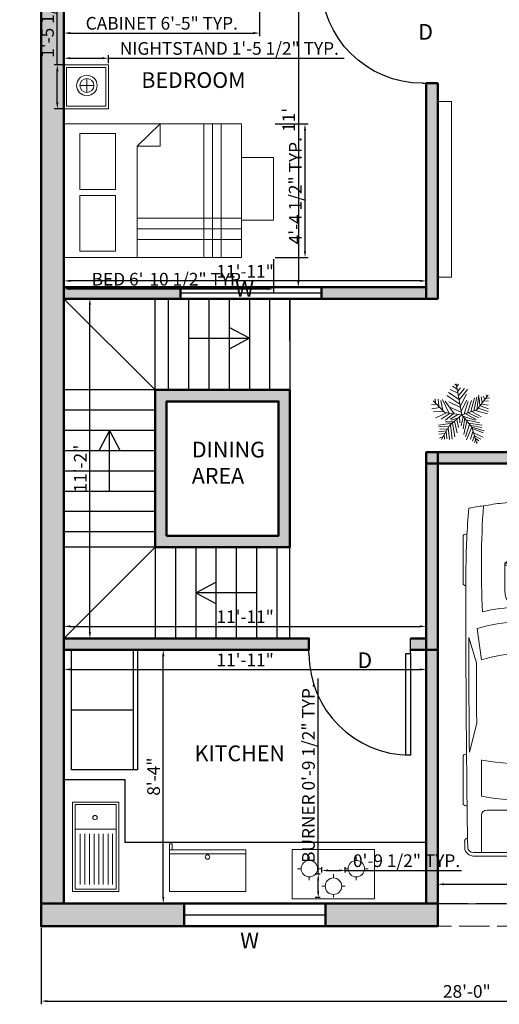
# Model space of a CAD drawing. Units: inches. Extents: x 2227 to 2709, y 1385 to 2029.
# Tile 1 of 4: x 2282 to 2472, y 1385 to 1773. Entities that reach past the tile are written whole.
import ezdxf

# ---------------------------------------------------------------- set-up
doc = ezdxf.new("R2010")
doc.units = ezdxf.units.IN
doc.linetypes.add('ACAD_ISO02W100', pattern=[15, 12, -3])
for name, color, linetype, lineweight in [('A-ANNO-DIMS', 1, 'Continuous', 18), ('A-ANNO-TEXT', 30, 'Continuous', 18), ('A-AREA-IDEN', 30, 'Continuous', 25), ('A-EQPM', 9, 'Continuous', 18), ('A-FLOR-CASE', 50, 'Continuous', 25), ('A-FLOR-FIXT', 9, 'Continuous', 18), ('A-FLOR-STRS', 7, 'Continuous', 25), ('A-FLOR-THRE', 8, 'ACAD_ISO02W100', 18), ('A-FURN', 50, 'Continuous', 18), ('A-SITE-VEHI', 8, 'Continuous', 13), ('A-WALL-PATT', 252, 'Continuous', 13), ('BED', 50, 'Continuous', 18), ('DOOR', 130, 'Continuous', 25), ('TREE', 80, 'Continuous', 13), ('WALL', 160, 'Continuous', 50), ('WIND', 40, 'Continuous', 25)]:
    doc.layers.add(name, color=color, linetype=linetype, lineweight=lineweight)
doc.styles.get("Standard").update_dxf_attribs({"font": 'arial.ttf'})
doc.dimstyles.new('ISO-25', dxfattribs={"dimtxt": 5, "dimasz": 2.5, "dimexe": 1.25, "dimexo": 0.625, "dimtad": 1, "dimdec": 0, "dimlunit": 4, "dimtxsty": 'Standard', "dimcen": 2.5, "dimadec": 0, "dimazin": 0, "dimtfac": 1, "dimtdec": 0, "dimtmove": 0, "dimatfit": 3, "dimfxl": 1, "dimarcsym": 0})

# ---------------------------------------------------------------- blocks, each defined once
blk = doc.blocks.new('*U8')
for p, q in [((21.1, 37.41), (21.1, 36.83)), ((46.55, 38.89), (22.35, 38.89)), ((47.8, 37.39), (47.8, 37.41)), ((87.99, 31.87), (74.76, 35.92)), ((135.45, 37.07), (135.45, 37.41)), ((136.7, 38.89), (160.9, 38.89)), ((162.15, 37.41), (162.15, 36.77)), ((70.03, 31.54), (86.41, 29.35)), ((134.31, 35.6), (119.29, 31.78)), ((186.47, -33.5), (186.47, 33.5)), ((188.4, -32.76), (188.4, 32.76)), ((138.42, 29.35), (157.25, 29.35)), ((164.52, 26.39), (164.52, -26.39)), ((186.47, 29.35), (167.01, 29.35)), ((32.27, 11.63), (36.13, 17.17)), ((36.13, 17.17), (50.94, 17.17)), ((32.12, 9.51), (32.12, 11.15)), ((58.92, -10.77), (58.92, 10.77)), ((66.55, -10.53), (66.55, 10.53)), ((186.47, -10.53), (186.47, 10.53)), ((3.27, 6.13), (0.1, 0.41)), ((29.77, 9.51), (51.68, 9.51)), ((82.74, 8.5), (82.74, -8.5)), ((0, 0), (51.68, 0)), ((0.1, -0.41), (3.27, -6.13)), ((29.77, -9.51), (51.68, -9.51)), ((32.12, -9.51), (32.12, -11.15)), ((32.27, -11.63), (36.13, -17.17)), ((36.13, -17.17), (50.94, -17.17)), ((86.41, -29.35), (70.03, -31.54)), ((157.25, -29.35), (138.42, -29.35)), ((167.01, -29.35), (186.47, -29.35)), ((87.99, -31.87), (74.76, -35.92)), ((134.31, -35.6), (119.29, -31.78)), ((21.1, -37.41), (21.1, -36.83)), ((46.55, -38.89), (22.35, -38.89)), ((47.8, -37.39), (47.8, -37.41)), ((135.45, -37.07), (135.45, -37.41)), ((136.7, -38.89), (160.9, -38.89)), ((162.15, -37.41), (162.15, -36.77))]:
    blk.add_line(p, q)
for centre, major_axis, ratio, start_param, end_param in [((266.03, -27.52), (0, 313.31), 0.842304, 1.367076, 1.39176), ((41.19, -490.86), (0, 528.23), 0.842304, 0.00281, 0.075598), ((22.35, 37.41), (0, -1.48), 0.842304, 3.141593, 4.712389), ((64.48, -10555.62), (0, 10593.03), 0.842304, -0.013397, 0.002797), ((46.55, 37.41), (0, 1.48), 0.842304, -1.570796, 0), ((64.48, -10555.62), (0, -10591.55), 0.842304, 3.133765, 3.140441), ((136.7, 37.41), (0, -1.48), 0.842304, 3.141593, 4.712389), ((160.9, 37.41), (0, 1.48), 0.842304, -1.570796, 0), ((180.63, 35.84), (0, 2.22), 0.842304, -0.013017, 1.249894), ((64.48, -10556.36), (0, 10595.31), 0.842304, -0.013397, -0.013017), ((183.98, 33.5), (0, -2.96), 0.842304, 1.570796, 3.128196), ((183.98, 32.76), (0, -5.25), 0.842304, 1.570796, 3.128196), ((135.29, 5.39), (0, 81.77), 0.842304, 1.245306, 1.50788), ((95.79, -3666.35), (0, -3698.24), 0.842304, 3.134049, 3.144098), ((259.18, -27.52), (0, -305.3), 0.842304, 4.528606, 4.561838), ((37.47, -593.96), (0, -623.33), 0.842304, 3.096046, 3.200911), ((134.4, 5.39), (0, -89.78), 0.842304, 4.449482, 4.652344), ((149.6, 2.8), (0, -79.58), 0.842304, 4.372215, 4.640744), ((17.08, 0), (0, 147.02), 0.842304, 4.511394, 4.913384), ((35.91, 0), (0, 147.02), 0.842304, 4.511394, 4.913384), ((167.01, 26.39), (0, 2.96), 0.842304, 0, 1.570796), ((-204.49, 52.4), (0, -250.96), 0.842304, 1.385369, 1.434372), ((13.04, 17.01), (0, 27.42), 0.842304, 4.435146, 4.718221), ((14.2, 17.01), (0, 27.42), 0.842304, 4.435146, 4.718221), ((50.79, 13.34), (6.34, -0.36), 0.603834, -1.395552, 1.581315), ((32.75, 11.15), (0, 0.74), 0.842304, 0.879714, 1.570796), ((29.77, -46.66), (0, 56.17), 0.842304, 0, 0.590319), ((0.62, 0), (0, -0.74), 0.842304, 4.131459, 5.293319), ((29.77, 46.66), (0, 56.17), 0.842304, 2.551274, 3.141593), ((-204.49, -52.4), (0, 250.96), 0.842304, -1.434372, -1.385369), ((13.04, -17.01), (0, -27.42), 0.842304, 1.564964, 1.848039), ((14.2, -17.01), (0, -27.42), 0.842304, 1.564964, 1.848039), ((149.6, -2.8), (0, -79.58), 0.842304, -1.499151, -1.230623), ((32.75, -11.15), (0, -0.74), 0.842304, 4.712389, 5.403472), ((134.4, -5.39), (0, -89.78), 0.842304, -1.510751, -1.307889), ((135.29, -5.39), (0, -81.77), 0.842304, -1.50788, -1.245306), ((259.18, 27.52), (0, 305.3), 0.842304, 1.721348, 1.754579), ((266.03, 27.52), (0, 313.31), 0.842304, 1.749832, 1.774517), ((37.47, 593.96), (0, -623.33), 0.842304, -0.059319, 0.045547), ((167.01, -26.39), (0, -2.96), 0.842304, 4.712389, 6.283185), ((64.48, 10555.62), (0, -10591.55), 0.842304, 0.001152, 0.007828), ((95.79, 3666.35), (0, -3698.24), 0.842304, -0.002505, 0.007544), ((183.98, -33.5), (0, 2.96), 0.842304, 3.15499, 4.712389), ((183.98, -32.76), (0, -5.25), 0.842304, 0.013397, 1.570796), ((41.19, 490.86), (0, -528.23), 0.842304, -0.075598, -0.00281), ((22.35, -37.41), (0, 1.48), 0.842304, 1.570796, 3.141593), ((64.48, 10555.62), (0, 10593.03), 0.842304, 3.138796, 3.15499), ((46.55, -37.41), (0, -1.48), 0.842304, 0, 1.570796), ((136.7, -37.41), (0, -1.48), 0.842304, -1.570796, 0), ((160.9, -37.41), (0, 1.48), 0.842304, 3.141593, 4.712389), ((180.63, -35.84), (0, -2.22), 0.842304, -1.249894, 0.013017), ((64.48, 10556.36), (0, 10595.31), 0.842304, 3.15461, 3.15499)]:
    blk.add_ellipse(centre, major_axis=major_axis, ratio=ratio, start_param=start_param, end_param=end_param)
at = {"extrusion": (0, 0, -1)}
blk.add_ellipse((50.79, -13.34), major_axis=(6.34, 0.36), ratio=0.603834, start_param=-1.395552, end_param=1.581315, dxfattribs=at)
blk = doc.blocks.new('*U2')
for p, q in [((0, 0), (0, -6)), ((40, 0), (40, -6))]:
    blk.add_line(p, q)
blk.add_lwpolyline([(0, 0), (0, 40), (1.75, 40), (1.75, 0)], close=True)
blk.add_arc((0, 0), 40, 0, 90)
blk = doc.blocks.new('*U6')
for p, q in [((-10.186, 53.64), (-13.084, 55.962)), ((0, 0), (-10.5, 57)), ((-9.099, 51.782), (-6.563, 55.962)), ((-5.114, 28.097), (-24.676, 40.636)), ((-7.288, 39.707), (-21.778, 46.673)), ((-8.737, 47.138), (-17.069, 52.711)), ((-7.65, 43.423), (-2.578, 49.46)), ((-5.839, 35.992), (4.667, 48.067)), ((-5.114, 27.632), (10.463, 46.673)), ((-2.941, 16.486), (8.652, 37.85)), ((44.153, 36.456), (45.239, 32.741)), ((-47.498, 19.737), (-55.83, 18.344)), ((-31.5, 4.5), (-52.5, 25.5)), ((-48.585, 21.131), (-49.309, 29.026)), ((-43.513, 28.561), (-42.427, 15.558)), ((-38.442, 26.239), (-34.819, 7.663)), ((-35.544, 28.097), (-24.314, 3.947)), ((-14.533, 2.09), (-30.834, 25.31)), ((-3.665, 19.273), (-27.574, 35.527)), ((-24.314, 23.917), (-2.941, 13.7)), ((-1.129, 6.734), (9.014, 26.704)), ((3.942, 1.625), (11.187, 24.381)), ((10.101, 3.483), (17.708, 26.239)), ((16.259, 5.805), (23.142, 31.348)), ((22.055, 7.198), (27.489, 32.277)), ((27, 9), (48, 36)), ((27.127, 9.056), (31.112, 35.992)), ((31.836, 30.883), (32.561, 16.486)), ((35.096, 32.741), (37.27, 22.524)), ((36.183, 19.737), (48.137, 17.88)), ((38.719, 34.134), (41.979, 28.561)), ((40.53, 25.775), (48.862, 24.846)), ((43.791, 29.954), (51.036, 30.883)), ((-40.615, 13.7), (-55.105, 10.913)), ((-33.37, 6.269), (-52.207, 5.34)), ((-28.299, 3.483), (-47.86, -5.805)), ((-21.416, 3.018), (-38.079, -8.128)), ((0, 0), (-31.5, 4.5)), ((-15.982, 2.09), (-30.11, -9.521)), ((0, 0), (-22.5, -19.5)), ((-6.563, 1.161), (-21.416, -8.128)), ((-20.691, 13.7), (-1.129, 4.876)), ((0, 0), (27, 9)), ((0, 0), (18, -22.5)), ((6.478, 1.625), (26.04, -8.592)), ((11.187, 3.483), (30.749, -5.805)), ((18.07, 5.805), (35.096, -3.483)), ((24.229, 7.663), (46.688, 1.625)), ((29.662, 12.307), (48.137, 6.269)), ((33.285, 16.486), (48.862, 10.913)), ((-17.431, -15.094), (-42.789, -18.809)), ((-15.257, -12.772), (-30.11, -12.772)), ((-6.563, -5.805), (-19.967, -9.985)), ((-17.069, -15.094), (-12.721, -40.172)), ((-13.446, -11.378), (-8.737, -32.741)), ((-9.461, -8.592), (-6.201, -23.453)), ((-4.752, -3.483), (-3.665, -14.629)), ((2.493, -3.019), (-1.491, -20.202)), ((1.769, -2.555), (24.229, -9.521)), ((5.029, -6.27), (2.131, -25.775)), ((9.014, -11.378), (3.58, -35.992)), ((14.085, -16.951), (6.478, -40.172)), ((7.565, -9.056), (32.198, -14.629)), ((12.274, -15.094), (36.907, -18.809)), ((-28.299, -29.026), (-42.789, -31.348)), ((-24.314, -21.596), (-42.427, -22.06)), ((-30.834, -34.135), (-42.427, -35.528)), ((-26.849, -26.24), (-40.253, -25.775)), ((-22.5, -19.5), (-37.5, -45)), ((-29.023, -30.884), (-27.936, -43.887)), ((-25.038, -23.918), (-22.865, -45.281)), ((-20.691, -18.345), (-17.793, -44.352)), ((18.07, -22.524), (8.289, -45.745)), ((20.244, -30.419), (15.897, -44.816)), ((16.259, -19.738), (36.183, -22.989)), ((18, -22.5), (27, -52.5)), ((18.433, -22.524), (40.53, -29.026)), ((19.157, -25.311), (38.719, -33.206)), ((21.331, -32.741), (39.081, -40.636)), ((-34.457, -39.708), (-40.978, -42.494)), ((-32.646, -36.921), (-31.921, -44.352)), ((22.78, -37.85), (19.519, -48.532)), ((22.78, -38.314), (34.372, -44.816)), ((24.591, -45.745), (23.142, -50.854)), ((24.591, -43.423), (30.749, -47.603)), ((26.764, -49.925), (28.213, -50.854))]:
    blk.add_line(p, q)
blk = doc.blocks.new('*D21')
at = {"layer": 'A-ANNO-DIMS', "color": 0, "lineweight": -2, "transparency": 16777216}
for p, q in [((2300.34, 1799.33), (2393.46, 1799.33)), ((2392.21, 1796.83), (2392.21, 1669.83)), ((2300.34, 1667.33), (2393.46, 1667.33))]:
    blk.add_line(p, q, dxfattribs=at)
at = {"layer": 'A-ANNO-DIMS', "color": 0, "lineweight": 100, "transparency": 16777216}
for points in [[(2391.79, 1796.83), (2392.62, 1796.83), (2392.21, 1799.33)], [(2391.79, 1669.83), (2392.62, 1669.83), (2392.21, 1667.33)]]:
    blk.add_solid(points, dxfattribs=at)
at = {"layer": 'Defpoints', "color": 0, "lineweight": 100, "transparency": 16777216}
for p in [(2299.71, 1799.33), (2299.71, 1667.33), (2392.21, 1667.33)]:
    blk.add_point(p, dxfattribs=at)
at = {"layer": 'A-ANNO-DIMS', "color": 0, "transparency": 16777216, "insert": (2389.07, 1733.33), "char_height": 5, "attachment_point": 5, "rotation": 90}
blk.add_mtext("11'", dxfattribs=at)
blk = doc.blocks.new('*D22')
at = {"layer": 'A-ANNO-DIMS', "color": 0, "lineweight": -2, "transparency": 16777216}
for p, q in [((2299.71, 1667.96), (2299.71, 1671.09)), ((2440.21, 1669.84), (2302.21, 1669.84)), ((2442.71, 1667.96), (2442.71, 1671.09))]:
    blk.add_line(p, q, dxfattribs=at)
at = {"layer": 'A-ANNO-DIMS', "color": 0, "lineweight": 100, "transparency": 16777216}
for points in [[(2302.21, 1670.26), (2302.21, 1669.42), (2299.71, 1669.84)], [(2440.21, 1670.26), (2440.21, 1669.42), (2442.71, 1669.84)]]:
    blk.add_solid(points, dxfattribs=at)
at = {"layer": 'Defpoints', "color": 0, "lineweight": 100, "transparency": 16777216}
for p in [(2299.71, 1669.84), (2299.71, 1667.33), (2442.71, 1667.33)]:
    blk.add_point(p, dxfattribs=at)
at = {"layer": 'A-ANNO-DIMS', "color": 0, "transparency": 16777216, "insert": (2371.21, 1672.98), "char_height": 5, "attachment_point": 5}
blk.add_mtext('11\'-11"', dxfattribs=at)
blk = doc.blocks.new('*D23')
at = {"layer": 'A-ANNO-DIMS', "color": 0, "lineweight": -2, "transparency": 16777216}
for p, q in [((2300.34, 1662.83), (2311.19, 1662.83)), ((2309.94, 1531.33), (2309.94, 1660.33)), ((2300.34, 1528.83), (2311.19, 1528.83))]:
    blk.add_line(p, q, dxfattribs=at)
at = {"layer": 'A-ANNO-DIMS', "color": 0, "lineweight": 100, "transparency": 16777216}
for points in [[(2309.52, 1660.33), (2310.35, 1660.33), (2309.94, 1662.83)], [(2309.52, 1531.33), (2310.35, 1531.33), (2309.94, 1528.83)]]:
    blk.add_solid(points, dxfattribs=at)
at = {"layer": 'Defpoints', "color": 0, "lineweight": 100, "transparency": 16777216}
for p in [(2299.71, 1662.83), (2309.94, 1662.83), (2299.71, 1528.83)]:
    blk.add_point(p, dxfattribs=at)
at = {"layer": 'A-ANNO-DIMS', "color": 0, "transparency": 16777216, "insert": (2306.8, 1595.83), "char_height": 5, "attachment_point": 5, "rotation": 90}
blk.add_mtext('11\'-2"', dxfattribs=at)
blk = doc.blocks.new('*D24')
at = {"layer": 'A-ANNO-DIMS', "color": 0, "lineweight": -2, "transparency": 16777216}
for p, q in [((2299.71, 1529.46), (2299.71, 1534.84)), ((2442.71, 1529.46), (2442.71, 1534.84)), ((2302.21, 1533.59), (2440.21, 1533.59))]:
    blk.add_line(p, q, dxfattribs=at)
at = {"layer": 'A-ANNO-DIMS', "color": 0, "lineweight": 100, "transparency": 16777216}
for points in [[(2302.21, 1534.01), (2302.21, 1533.18), (2299.71, 1533.59)], [(2440.21, 1534.01), (2440.21, 1533.18), (2442.71, 1533.59)]]:
    blk.add_solid(points, dxfattribs=at)
at = {"layer": 'Defpoints', "color": 0, "lineweight": 100, "transparency": 16777216}
for p in [(2442.71, 1533.59), (2299.71, 1528.83), (2442.71, 1528.83)]:
    blk.add_point(p, dxfattribs=at)
at = {"layer": 'A-ANNO-DIMS', "color": 0, "transparency": 16777216, "insert": (2371.21, 1536.73), "char_height": 5, "attachment_point": 5}
blk.add_mtext('11\'-11"', dxfattribs=at)
blk = doc.blocks.new('*D25')
at = {"layer": 'A-ANNO-DIMS', "color": 0, "lineweight": -2, "transparency": 16777216}
for p, q in [((2299.71, 1523.71), (2299.71, 1515.35)), ((2442.71, 1523.71), (2442.71, 1515.35)), ((2302.21, 1516.6), (2440.21, 1516.6))]:
    blk.add_line(p, q, dxfattribs=at)
at = {"layer": 'A-ANNO-DIMS', "color": 0, "lineweight": 100, "transparency": 16777216}
for points in [[(2302.21, 1517.02), (2302.21, 1516.18), (2299.71, 1516.6)], [(2440.21, 1517.02), (2440.21, 1516.18), (2442.71, 1516.6)]]:
    blk.add_solid(points, dxfattribs=at)
at = {"layer": 'Defpoints', "color": 0, "lineweight": 100, "transparency": 16777216}
for p in [(2299.71, 1524.33), (2442.71, 1524.33), (2442.71, 1516.6)]:
    blk.add_point(p, dxfattribs=at)
at = {"layer": 'A-ANNO-DIMS', "color": 0, "transparency": 16777216, "insert": (2371.21, 1519.74), "char_height": 5, "attachment_point": 5}
blk.add_mtext('11\'-11"', dxfattribs=at)
blk = doc.blocks.new('*D26')
at = {"layer": 'A-ANNO-DIMS', "color": 0, "lineweight": -2, "transparency": 16777216}
for p, q in [((2300.34, 1524.33), (2340.16, 1524.33)), ((2338.91, 1426.83), (2338.91, 1521.83)), ((2300.34, 1424.33), (2340.16, 1424.33))]:
    blk.add_line(p, q, dxfattribs=at)
at = {"layer": 'A-ANNO-DIMS', "color": 0, "lineweight": 100, "transparency": 16777216}
for points in [[(2338.49, 1521.83), (2339.33, 1521.83), (2338.91, 1524.33)], [(2338.49, 1426.83), (2339.33, 1426.83), (2338.91, 1424.33)]]:
    blk.add_solid(points, dxfattribs=at)
at = {"layer": 'Defpoints', "color": 0, "lineweight": 100, "transparency": 16777216}
for p in [(2299.71, 1524.33), (2338.91, 1524.33), (2299.71, 1424.33)]:
    blk.add_point(p, dxfattribs=at)
at = {"layer": 'A-ANNO-DIMS', "color": 0, "transparency": 16777216, "insert": (2335.73, 1474.33), "char_height": 5, "attachment_point": 5, "rotation": 90}
blk.add_mtext('8\'-4"', dxfattribs=at)
blk = doc.blocks.new('*D27')
at = {"layer": 'A-ANNO-DIMS', "color": 0, "lineweight": -2, "transparency": 16777216}
for p, q in [((2447.21, 1424.96), (2447.21, 1433.13)), ((2617.71, 1424.96), (2617.71, 1433.13)), ((2449.71, 1431.88), (2615.21, 1431.88))]:
    blk.add_line(p, q, dxfattribs=at)
at = {"layer": 'A-ANNO-DIMS', "color": 0, "lineweight": 100, "transparency": 16777216}
for points in [[(2449.71, 1432.3), (2449.71, 1431.46), (2447.21, 1431.88)], [(2615.21, 1432.3), (2615.21, 1431.46), (2617.71, 1431.88)]]:
    blk.add_solid(points, dxfattribs=at)
at = {"layer": 'Defpoints', "color": 0, "lineweight": 100, "transparency": 16777216}
for p in [(2617.71, 1431.88), (2447.21, 1424.33), (2617.71, 1424.33)]:
    blk.add_point(p, dxfattribs=at)
at = {"layer": 'A-ANNO-DIMS', "color": 0, "transparency": 16777216, "insert": (2532.46, 1435.06), "char_height": 5, "attachment_point": 5}
blk.add_mtext('14\'-3"', dxfattribs=at)
blk = doc.blocks.new('*D28')
at = {"layer": 'A-ANNO-DIMS', "color": 0, "lineweight": -2, "transparency": 16777216}
for p, q in [((2448.57, 1597.83), (2527.6, 1597.5)), ((2525.63, 1426.5), (2526.34, 1595)), ((2447.84, 1424.33), (2526.87, 1424))]:
    blk.add_line(p, q, dxfattribs=at)
at = {"layer": 'A-ANNO-DIMS', "color": 0, "lineweight": 100, "transparency": 16777216}
for points in [[(2525.92, 1595), (2526.75, 1595), (2526.35, 1597.5)], [(2525.21, 1426.5), (2526.04, 1426.5), (2525.62, 1424)]]:
    blk.add_solid(points, dxfattribs=at)
at = {"layer": 'Defpoints', "color": 0, "lineweight": 100, "transparency": 16777216}
for p in [(2447.95, 1597.83), (2526.35, 1597.5), (2447.21, 1424.33)]:
    blk.add_point(p, dxfattribs=at)
at = {"layer": 'A-ANNO-DIMS', "color": 0, "transparency": 16777216, "insert": (2522.8, 1510.77), "char_height": 5, "attachment_point": 5, "rotation": 89.7584}
blk.add_mtext('14\'-6"', dxfattribs=at)
blk = doc.blocks.new('BED-DOUBLE')
for p, q in [((37.96, 0), (28.86, -8.71)), ((37.96, -8.71), (37.96, 0)), ((55.17, -52.67), (55.17, 0)), ((58.68, -52.67), (58.68, 0)), ((62.04, -52.67), (62.04, 0)), ((28.86, -52.67), (28.86, -8.71)), ((28.86, -8.71), (37.96, -8.71)), ((28.86, -37.1), (70.02, -37.1)), ((28.86, -41.31), (70.02, -41.31)), ((28.86, -45.51), (70.02, -45.51))]:
    blk.add_line(p, q)
for points in [[(0, 0), (70.02, 0), (70.02, -52.67), (0, -52.67)], [(6.26, -25.79), (20.3, -25.79), (20.3, -3.78), (6.26, -3.78)], [(70.02, -38), (82.72, -38), (82.72, -13.23), (70.02, -13.23)], [(6.26, -50.18), (20.3, -50.18), (20.3, -28.17), (6.26, -28.17)]]:
    blk.add_lwpolyline(points, close=True)
blk = doc.blocks.new('NIGHTSTAND')
for p, q in [((9.06, 6.42), (9.06, 11.97)), ((6.28, 9.2), (11.83, 9.2))]:
    blk.add_line(p, q)
for points in [[(0, 0), (17.54, 0), (17.54, 17.32), (0, 17.32)], [(1, 1), (16.54, 1), (16.54, 16.32), (1, 16.32)]]:
    blk.add_lwpolyline(points, close=True)
for radius in [4.05, 2.77]:
    blk.add_circle((9.06, 9.2), radius)
blk = doc.blocks.new('STAIR-DIRECTION')
for p, q in [((0, 0), (8, 4.23)), ((24, 0), (0, 0)), ((0, 0), (8, -4.23))]:
    blk.add_line(p, q)
blk = doc.blocks.new('COOKTOP-BURNER')
for p, q in [((0, 3.25), (0, 4.8)), ((-3.25, 0), (-4.62, 0)), ((0, -3.25), (0, -4.52)), ((3.25, 0), (4.66, 0))]:
    blk.add_line(p, q)
blk.add_circle((0, 0), 3.25)
blk = doc.blocks.new('*D37')
at = {"layer": 'A-ANNO-DIMS', "color": 0, "lineweight": -2, "transparency": 16777216}
for p, q in [((2299.71, 1678.44), (2299.71, 1665.41)), ((2382.43, 1678.44), (2382.43, 1665.41)), ((2302.21, 1666.66), (2379.93, 1666.66))]:
    blk.add_line(p, q, dxfattribs=at)
at = {"layer": 'A-ANNO-DIMS', "color": 0, "lineweight": 100, "transparency": 16777216}
for points in [[(2302.21, 1667.07), (2302.21, 1666.24), (2299.71, 1666.66)], [(2379.93, 1667.07), (2379.93, 1666.24), (2382.43, 1666.66)]]:
    blk.add_solid(points, dxfattribs=at)
at = {"layer": 'Defpoints', "color": 0, "lineweight": 100, "transparency": 16777216}
for p in [(2299.71, 1679.06), (2382.43, 1679.06), (2382.43, 1666.66)]:
    blk.add_point(p, dxfattribs=at)
at = {"layer": 'A-ANNO-DIMS', "color": 0, "transparency": 16777216, "insert": (2341.07, 1669.87), "char_height": 5, "attachment_point": 5}
blk.add_mtext('BED 6\'-10 1/2" TYP.', dxfattribs=at)
blk = doc.blocks.new('*D38')
at = {"layer": 'A-ANNO-DIMS', "color": 0, "lineweight": -2, "transparency": 16777216}
for p, q in [((2383.06, 1731.73), (2396.09, 1731.73)), ((2394.84, 1681.56), (2394.84, 1729.23)), ((2383.06, 1679.06), (2396.09, 1679.06))]:
    blk.add_line(p, q, dxfattribs=at)
at = {"layer": 'A-ANNO-DIMS', "color": 0, "lineweight": 100, "transparency": 16777216}
for points in [[(2394.42, 1729.23), (2395.25, 1729.23), (2394.84, 1731.73)], [(2394.42, 1681.56), (2395.25, 1681.56), (2394.84, 1679.06)]]:
    blk.add_solid(points, dxfattribs=at)
at = {"layer": 'Defpoints', "color": 0, "lineweight": 100, "transparency": 16777216}
for p in [(2382.43, 1731.73), (2394.84, 1731.73), (2382.43, 1679.06)]:
    blk.add_point(p, dxfattribs=at)
at = {"layer": 'A-ANNO-DIMS', "color": 0, "transparency": 16777216, "insert": (2391.63, 1705.4), "char_height": 5, "attachment_point": 5, "rotation": 90}
blk.add_mtext('4\'-4 1/2" TYP.', dxfattribs=at)
blk = doc.blocks.new('*D39')
at = {"layer": 'A-ANNO-DIMS', "color": 0, "lineweight": -2, "transparency": 16777216}
for p, q in [((2299.71, 1778.54), (2299.71, 1766.33)), ((2376.93, 1778.54), (2376.93, 1766.33)), ((2302.21, 1767.58), (2374.43, 1767.58))]:
    blk.add_line(p, q, dxfattribs=at)
at = {"layer": 'A-ANNO-DIMS', "color": 0, "lineweight": 100, "transparency": 16777216}
for points in [[(2302.21, 1768), (2302.21, 1767.16), (2299.71, 1767.58)], [(2374.43, 1768), (2374.43, 1767.16), (2376.93, 1767.58)]]:
    blk.add_solid(points, dxfattribs=at)
at = {"layer": 'Defpoints', "color": 0, "lineweight": 100, "transparency": 16777216}
for p in [(2299.71, 1779.16), (2376.93, 1779.16), (2376.93, 1767.58)]:
    blk.add_point(p, dxfattribs=at)
at = {"layer": 'A-ANNO-DIMS', "color": 0, "transparency": 16777216, "insert": (2338.32, 1770.79), "char_height": 5, "attachment_point": 5}
blk.add_mtext('CABINET 6\'-5" TYP.', dxfattribs=at)
blk = doc.blocks.new('*D41')
at = {"layer": 'A-ANNO-DIMS', "color": 0, "lineweight": -2, "transparency": 16777216}
for p, q in [((2299.71, 1755.65), (2299.71, 1758.91)), ((2302.21, 1757.66), (2314.75, 1757.66)), ((2317.25, 1755.65), (2317.25, 1758.91)), ((2317.25, 1757.66), (2410.23, 1757.66))]:
    blk.add_line(p, q, dxfattribs=at)
at = {"layer": 'A-ANNO-DIMS', "color": 0, "lineweight": 100, "transparency": 16777216}
for points in [[(2302.21, 1758.07), (2302.21, 1757.24), (2299.71, 1757.66)], [(2314.75, 1758.07), (2314.75, 1757.24), (2317.25, 1757.66)]]:
    blk.add_solid(points, dxfattribs=at)
at = {"layer": 'Defpoints', "color": 0, "lineweight": 100, "transparency": 16777216}
for p in [(2317.25, 1757.66), (2299.71, 1755.03), (2317.25, 1755.03)]:
    blk.add_point(p, dxfattribs=at)
at = {"layer": 'A-ANNO-DIMS', "color": 0, "transparency": 16777216, "insert": (2364.99, 1760.87), "char_height": 5, "attachment_point": 5}
blk.add_mtext('NIGHTSTAND 1\'-5 1/2" TYP.', dxfattribs=at)
blk = doc.blocks.new('*D42')
at = {"layer": 'A-ANNO-DIMS', "color": 0, "lineweight": -2, "transparency": 16777216}
for p, q in [((2297.08, 1755.03), (2297.08, 1800.43)), ((2299.09, 1755.03), (2295.83, 1755.03)), ((2297.08, 1740.21), (2297.08, 1752.53)), ((2299.09, 1737.71), (2295.83, 1737.71))]:
    blk.add_line(p, q, dxfattribs=at)
at = {"layer": 'A-ANNO-DIMS', "color": 0, "lineweight": 100, "transparency": 16777216}
for points in [[(2296.67, 1752.53), (2297.5, 1752.53), (2297.08, 1755.03)], [(2296.67, 1740.21), (2297.5, 1740.21), (2297.08, 1737.71)]]:
    blk.add_solid(points, dxfattribs=at)
at = {"layer": 'Defpoints', "color": 0, "lineweight": 100, "transparency": 16777216}
for p in [(2297.08, 1755.03), (2299.71, 1755.03), (2299.71, 1737.71)]:
    blk.add_point(p, dxfattribs=at)
at = {"layer": 'A-ANNO-DIMS', "color": 0, "transparency": 16777216, "insert": (2293.87, 1778.98), "char_height": 5, "attachment_point": 5, "rotation": 90}
blk.add_mtext('1\'-5 1/2" TYP.', dxfattribs=at)
blk = doc.blocks.new('*D45')
at = {"layer": 'A-ANNO-DIMS', "color": 0, "lineweight": -2, "transparency": 16777216}
for p, q in [((2400.05, 1435.92), (2400.05, 1513.02)), ((2400.82, 1435.92), (2398.8, 1435.92)), ((2400.05, 1429.1), (2400.05, 1433.42)), ((2400.82, 1426.6), (2398.8, 1426.6))]:
    blk.add_line(p, q, dxfattribs=at)
at = {"layer": 'A-ANNO-DIMS', "color": 0, "lineweight": 100, "transparency": 16777216}
for points in [[(2399.63, 1433.42), (2400.46, 1433.42), (2400.05, 1435.92)], [(2399.63, 1429.1), (2400.46, 1429.1), (2400.05, 1426.6)]]:
    blk.add_solid(points, dxfattribs=at)
at = {"layer": 'Defpoints', "color": 0, "lineweight": 100, "transparency": 16777216}
for p in [(2400.05, 1435.92), (2401.45, 1435.92), (2401.45, 1426.6)]:
    blk.add_point(p, dxfattribs=at)
at = {"layer": 'A-ANNO-DIMS', "color": 0, "transparency": 16777216, "insert": (2396.84, 1475.72), "char_height": 5, "attachment_point": 5, "rotation": 90}
blk.add_mtext('BURNER 0\'-9 1/2" TYP.', dxfattribs=at)
blk = doc.blocks.new('*D46')
at = {"layer": 'A-ANNO-DIMS', "color": 0, "lineweight": -2, "transparency": 16777216}
for p, q in [((2401.45, 1436.55), (2401.45, 1438.57)), ((2403.95, 1437.32), (2408.23, 1437.32)), ((2410.73, 1436.55), (2410.73, 1438.57)), ((2410.73, 1437.32), (2456.61, 1437.32))]:
    blk.add_line(p, q, dxfattribs=at)
at = {"layer": 'A-ANNO-DIMS', "color": 0, "lineweight": 100, "transparency": 16777216}
for points in [[(2403.95, 1437.74), (2403.95, 1436.91), (2401.45, 1437.32)], [(2408.23, 1437.74), (2408.23, 1436.91), (2410.73, 1437.32)]]:
    blk.add_solid(points, dxfattribs=at)
at = {"layer": 'Defpoints', "color": 0, "lineweight": 100, "transparency": 16777216}
for p in [(2410.73, 1437.32), (2401.45, 1435.92), (2410.73, 1435.92)]:
    blk.add_point(p, dxfattribs=at)
at = {"layer": 'A-ANNO-DIMS', "color": 0, "transparency": 16777216, "insert": (2434.92, 1440.53), "char_height": 5, "attachment_point": 5}
blk.add_mtext('0\'-9 1/2" TYP.', dxfattribs=at)
blk = doc.blocks.new('*D47')
at = {"layer": 'A-ANNO-DIMS', "color": 0, "lineweight": -2, "transparency": 16777216}
for p, q in [((2290.71, 1414.71), (2290.71, 1384.53)), ((2626.71, 1414.71), (2626.71, 1384.53)), ((2293.21, 1385.78), (2624.21, 1385.78))]:
    blk.add_line(p, q, dxfattribs=at)
at = {"layer": 'A-ANNO-DIMS', "color": 0, "lineweight": 100, "transparency": 16777216}
for points in [[(2293.21, 1386.2), (2293.21, 1385.37), (2290.71, 1385.78)], [(2624.21, 1386.2), (2624.21, 1385.37), (2626.71, 1385.78)]]:
    blk.add_solid(points, dxfattribs=at)
at = {"layer": 'Defpoints', "color": 0, "lineweight": 100, "transparency": 16777216}
for p in [(2290.71, 1415.33), (2626.71, 1415.33), (2626.71, 1385.78)]:
    blk.add_point(p, dxfattribs=at)
at = {"layer": 'A-ANNO-DIMS', "color": 0, "transparency": 16777216, "insert": (2458.71, 1388.96), "char_height": 5, "attachment_point": 5}
blk.add_mtext('28\'-0"', dxfattribs=at)

msp = doc.modelspace()

# ---------------------------------------------------------------- hatches: boundary and pattern name
at = {"layer": 'A-WALL-PATT'}
h = msp.add_hatch(color=256, dxfattribs=at)
h.dxf.hatch_style = 1
h.paths.add_polyline_path([(2538.21, 1991.33), (2290.71, 1991.33), (2290.71, 1982.33), (2299.71, 1982.33), (2538.21, 1982.33)])
h.paths.add_polyline_path([(2299.71, 1982.33), (2290.71, 1982.33), (2290.71, 1424.33), (2299.71, 1424.33)])
h.paths.add_polyline_path([(2347.13, 1424.33), (2290.71, 1424.33), (2290.71, 1415.33), (2347.13, 1415.33)])
h.paths.add_polyline_path([(2447.21, 1424.33), (2402.93, 1424.33), (2402.93, 1415.33), (2447.21, 1415.33)])
h.paths.add_polyline_path([(2447.21, 1597.83), (2442.71, 1597.83), (2442.71, 1424.33), (2447.21, 1424.33)])
h.paths.add_polyline_path([(2396.41, 1528.83), (2299.71, 1528.83), (2299.71, 1524.33), (2396.41, 1524.33)])
h.paths.add_polyline_path([(2442.71, 1528.83), (2436.41, 1528.83), (2436.41, 1524.33), (2442.71, 1524.33)])
h.paths.add_polyline_path([(2345.64, 1667.33), (2299.71, 1667.33), (2299.71, 1662.83), (2345.64, 1662.83)])
h.paths.add_polyline_path([(2447.21, 1747.77), (2442.71, 1747.77), (2442.71, 1662.83), (2447.21, 1662.83)])
h.paths.add_polyline_path([(2442.71, 1667.33), (2401.29, 1667.33), (2401.29, 1662.83), (2442.71, 1662.83)])
h.paths.add_polyline_path([(2447.21, 1803.83), (2299.71, 1803.83), (2299.71, 1799.33), (2447.21, 1799.33)])
h.paths.add_polyline_path([(2447.21, 1799.33), (2442.71, 1799.33), (2442.71, 1787.77), (2447.21, 1787.77)])
h.paths.add_polyline_path([(2394.45, 1851.83), (2389.95, 1851.83), (2389.95, 1803.83), (2394.45, 1803.83)])
h.paths.add_polyline_path([(2327.17, 1851.83), (2322.67, 1851.83), (2322.67, 1840.2), (2327.17, 1840.2)])
h.paths.add_polyline_path([(2327.17, 1815.42), (2322.67, 1815.42), (2322.67, 1803.83), (2327.17, 1803.83)])
h.paths.add_polyline_path([(2397.41, 1856.33), (2299.71, 1856.33), (2299.71, 1851.83), (2397.41, 1851.83)])
h.paths.add_polyline_path([(2447.21, 1856.33), (2437.41, 1856.33), (2437.41, 1851.83), (2447.21, 1851.83)])
h.paths.add_polyline_path([(2447.21, 1934.33), (2442.71, 1934.33), (2442.71, 1856.33), (2447.21, 1856.33)])
h.paths.add_polyline_path([(2459.62, 1856.33), (2447.21, 1856.33), (2447.21, 1851.83), (2459.62, 1851.83)])
h.paths.add_polyline_path([(2498.21, 1856.33), (2494.53, 1856.33), (2494.53, 1851.83), (2498.21, 1851.83)])
h.paths.add_polyline_path([(2462.23, 1934.33), (2447.21, 1934.33), (2447.21, 1929.83), (2462.23, 1929.83)])
h.paths.add_polyline_path([(2507.32, 1934.33), (2483.3, 1934.33), (2483.3, 1929.83), (2507.32, 1929.83)])
h.paths.add_polyline_path([(2542.71, 1947.66), (2538.21, 1947.66), (2538.21, 1934.33), (2542.71, 1934.33)])
h.paths.add_polyline_path([(2544.78, 1934.33), (2536.35, 1934.33), (2536.35, 1929.83), (2544.78, 1929.83)])
h.paths.add_polyline_path([(2542.71, 1982.33), (2538.21, 1982.33), (2538.21, 1971.57), (2542.71, 1971.57)])
h.paths.add_polyline_path([(2346.6, 1815.57), (2382.82, 1815.57), (2382.82, 1838.66), (2346.6, 1838.66)], flags=9)
h.paths.add_polyline_path([(2457.86, 1902.08), (2494.08, 1902.08), (2494.08, 1925.17), (2457.86, 1925.17)], flags=9)
h.paths.add_polyline_path([(2500.39, 1690.49), (2545.31, 1690.49), (2545.31, 1713.58), (2500.39, 1713.58)], flags=9)
h.paths.add_polyline_path([(2528.08, 1476.92), (2562.42, 1476.92), (2562.42, 1489.69), (2528.08, 1489.69)], flags=9)
h.paths.add_polyline_path([(2349.07, 1476.93), (2390.15, 1476.93), (2390.15, 1489.69), (2349.07, 1489.69)], flags=9)
h.paths.add_polyline_path([(2347.99, 1586.39), (2381.37, 1586.39), (2381.37, 1609.48), (2347.99, 1609.48)], flags=9)
h.paths.add_polyline_path([(2328.07, 1742.46), (2375.88, 1742.46), (2375.88, 1755.23), (2328.07, 1755.23)], flags=9)
h.paths.add_polyline_path([(2556.42, 1893.75), (2604.23, 1893.75), (2604.23, 1906.51), (2556.42, 1906.51)], flags=9)
h.paths.add_polyline_path([(2323.02, 1893.88), (2370.83, 1893.88), (2370.83, 1906.64), (2323.02, 1906.64)], flags=9)
h.paths.add_polyline_path([(2562.19, 1958.77), (2598.41, 1958.77), (2598.41, 1981.86), (2562.19, 1981.86)], flags=9)
h.paths.add_polyline_path([(2482.23, 1953.14), (2507.92, 1953.14), (2507.92, 1965.9), (2482.23, 1965.9)], flags=9)
h = msp.add_hatch(color=256, dxfattribs=at)
h.dxf.hatch_style = 1
h.paths.add_polyline_path([(2388.88, 1626.83), (2335.71, 1626.83), (2335.71, 1564.83), (2388.88, 1564.83)])
h.paths.add_polyline_path([(2384.38, 1569.33), (2340.21, 1569.33), (2340.21, 1622.33), (2384.38, 1622.33)], flags=16)
h.paths.add_polyline_path([(2347.99, 1586.39), (2381.37, 1586.39), (2381.37, 1609.48), (2347.99, 1609.48)], flags=8)
h = msp.add_hatch(color=256, dxfattribs=at)
h.dxf.hatch_style = 1
h.paths.add_polyline_path([(2476.5, 1602.33), (2447.21, 1602.33), (2447.21, 1597.83), (2476.5, 1597.83)])
h.paths.add_polyline_path([(2447.21, 1602.33), (2442.71, 1602.33), (2442.71, 1597.83), (2447.21, 1597.83)])

# ---------------------------------------------------------------- linework, layer by layer
at = {"layer": 'A-EQPM'}
msp.add_lwpolyline([(2422.24, 1445.64), (2389.77, 1445.64), (2389.77, 1426.13), (2422.24, 1426.13)], close=True, dxfattribs=at)
at = {"layer": 'A-FLOR-CASE'}
for p, q in [((2327.19, 1476.96), (2327.19, 1524.33)), ((2302.67, 1500.64), (2327.19, 1500.64)), ((2299.71, 1473.25), (2323.71, 1473.25)), ((2323.71, 1473.25), (2323.71, 1448.33)), ((2442.71, 1448.33), (2323.71, 1448.33)), ((2442.71, 1424.33), (2442.71, 1448.33))]:
    msp.add_line(p, q, dxfattribs=at)
msp.add_lwpolyline([(2302.67, 1524.33), (2328.68, 1524.33), (2328.68, 1476.96), (2302.67, 1476.96)], close=True, dxfattribs=at)
at = {"layer": 'A-FLOR-FIXT'}
for p, q in [((2304.1, 1453.55), (2320.31, 1453.55)), ((2306.15, 1431.78), (2306.15, 1451.79)), ((2307.95, 1431.78), (2307.95, 1451.79)), ((2309.75, 1431.78), (2309.75, 1451.79)), ((2311.63, 1431.78), (2311.63, 1451.79)), ((2313.43, 1431.78), (2313.43, 1451.79)), ((2315.23, 1431.78), (2315.23, 1451.79)), ((2317.1, 1431.78), (2317.1, 1451.79)), ((2318.82, 1431.78), (2318.82, 1451.79)), ((2341.33, 1443.87), (2371.43, 1443.87))]:
    msp.add_line(p, q, dxfattribs=at)
for points in [[(2303.1, 1464.27), (2321.31, 1464.27), (2321.31, 1429), (2303.1, 1429)], [(2304.1, 1463.27), (2320.31, 1463.27), (2320.31, 1430), (2304.1, 1430)], [(2341.33, 1445.4), (2342.37, 1445.4), (2342.37, 1447.87), (2341.33, 1447.87)], [(2341.33, 1445.4), (2371.43, 1445.4), (2371.43, 1428.96), (2341.33, 1428.96)]]:
    msp.add_lwpolyline(points, close=True, dxfattribs=at)
for centre, radius in [((2311.95, 1458.16), 0.873), ((2356.38, 1442.63), 0.877)]:
    msp.add_circle(centre, radius, dxfattribs=at)
at = {"layer": 'A-FLOR-STRS'}
for p, q in [((2335.71, 1626.83), (2299.71, 1662.83)), ((2335.71, 1626.83), (2335.71, 1662.83)), ((2340.88, 1662.83), (2340.88, 1626.83)), ((2348.88, 1662.83), (2348.88, 1626.83)), ((2356.88, 1662.83), (2356.88, 1626.83)), ((2364.88, 1662.83), (2364.88, 1626.83)), ((2372.88, 1662.83), (2372.88, 1626.83)), ((2380.88, 1662.83), (2380.88, 1626.83)), ((2388.88, 1646.34), (2388.88, 1662.83)), ((2388.88, 1662.83), (2388.88, 1626.83)), ((2335.71, 1626.83), (2299.71, 1626.83)), ((2388.88, 1626.83), (2335.71, 1626.83)), ((2335.71, 1626.83), (2335.71, 1564.83)), ((2388.88, 1564.83), (2388.88, 1626.83)), ((2335.71, 1618.83), (2299.71, 1618.83)), ((2335.71, 1610.83), (2299.71, 1610.83)), ((2335.71, 1602.83), (2299.71, 1602.83)), ((2335.71, 1594.83), (2299.71, 1594.83)), ((2335.71, 1586.83), (2299.71, 1586.83)), ((2335.71, 1578.83), (2299.71, 1578.83)), ((2335.71, 1570.83), (2299.71, 1570.83)), ((2335.71, 1564.83), (2299.71, 1564.83)), ((2335.71, 1564.83), (2299.71, 1528.83)), ((2388.88, 1564.83), (2335.71, 1564.83)), ((2335.71, 1564.83), (2335.71, 1528.83)), ((2343.71, 1564.83), (2343.71, 1528.83)), ((2351.71, 1564.83), (2351.71, 1528.83)), ((2359.71, 1564.83), (2359.71, 1528.83)), ((2367.71, 1564.83), (2367.71, 1528.83)), ((2375.71, 1564.83), (2375.71, 1528.83)), ((2383.71, 1564.83), (2383.71, 1528.83)), ((2388.88, 1528.83), (2388.88, 1564.83))]:
    msp.add_line(p, q, dxfattribs=at)
at = {"layer": 'A-FLOR-THRE'}
msp.add_lwpolyline([(2617.71, 1415.33), (2447.21, 1415.33), (2447.21, 1424.33), (2617.71, 1424.33)], close=True, dxfattribs=at)
at = {"layer": 'A-FURN'}
msp.add_lwpolyline([(2447.21, 1671.33), (2452.69, 1671.33), (2452.69, 1740.54), (2447.21, 1740.54)], close=True, dxfattribs=at)
at = {"layer": 'WALL'}
for p, q in [((2290.71, 1415.33), (2290.71, 1991.33)), ((2442.71, 1747.77), (2442.71, 1667.33)), ((2447.21, 1747.77), (2447.21, 1662.83)), ((2442.71, 1667.33), (2299.71, 1667.33)), ((2447.21, 1662.83), (2299.71, 1662.83)), ((2299.71, 1662.83), (2299.71, 1528.83)), ((2442.71, 1528.83), (2442.71, 1602.33)), ((2447.21, 1602.33), (2442.71, 1602.33)), ((2447.21, 1524.33), (2447.21, 1602.33)), ((2563.54, 1602.33), (2447.21, 1602.33)), ((2562.56, 1597.83), (2447.21, 1597.83)), ((2299.71, 1528.83), (2396.41, 1528.83)), ((2436.41, 1528.83), (2442.71, 1528.83)), ((2299.71, 1524.33), (2396.41, 1524.33)), ((2299.71, 1524.33), (2396.41, 1524.33)), ((2436.41, 1524.33), (2442.71, 1524.33)), ((2436.41, 1524.33), (2447.21, 1524.33)), ((2442.71, 1524.33), (2442.71, 1424.33)), ((2447.21, 1524.33), (2447.21, 1424.33)), ((2442.71, 1428.33), (2442.71, 1424.33)), ((2447.21, 1424.33), (2447.21, 1415.33)), ((2447.21, 1415.33), (2290.71, 1415.33))]:
    msp.add_line(p, q, dxfattribs=at)
for points in [[(2447.21, 1415.33), (2290.71, 1415.33), (2290.71, 1991.33), (2626.71, 1991.33), (2626.71, 1415.33), (2617.71, 1415.33)], [(2447.21, 1424.33), (2299.71, 1424.33), (2299.71, 1982.33), (2617.71, 1982.33), (2617.71, 1424.33)]]:
    msp.add_lwpolyline(points, dxfattribs=at)
for points in [[(2290.71, 1982.33), (2299.71, 1982.33), (2299.71, 1424.33), (2290.71, 1424.33)], [(2442.71, 1747.77), (2447.21, 1747.77), (2447.21, 1662.83), (2442.71, 1662.83)], [(2299.71, 1662.83), (2345.64, 1662.83), (2345.64, 1667.33), (2299.71, 1667.33)], [(2401.29, 1662.83), (2442.71, 1662.83), (2442.71, 1667.33), (2401.29, 1667.33)], [(2335.71, 1564.83), (2388.88, 1564.83), (2388.88, 1626.83), (2335.71, 1626.83)], [(2340.21, 1569.33), (2384.38, 1569.33), (2384.38, 1622.33), (2340.21, 1622.33)], [(2476.5, 1597.83), (2442.71, 1597.83), (2442.71, 1602.33), (2476.5, 1602.33)], [(2442.71, 1597.83), (2447.21, 1597.83), (2447.21, 1424.33), (2442.71, 1424.33)], [(2299.71, 1524.33), (2396.41, 1524.33), (2396.41, 1528.83), (2299.71, 1528.83)], [(2290.71, 1415.33), (2347.13, 1415.33), (2347.13, 1424.33), (2290.71, 1424.33)], [(2402.93, 1415.33), (2447.21, 1415.33), (2447.21, 1424.33), (2402.93, 1424.33)]]:
    msp.add_lwpolyline(points, close=True, dxfattribs=at)
at = {"layer": 'WIND'}
for p, q in [((2345.64, 1665.08), (2401.29, 1665.08)), ((2347.13, 1419.83), (2402.93, 1419.83))]:
    msp.add_line(p, q, dxfattribs=at)
for points in [[(2345.64, 1662.83), (2401.29, 1662.83), (2401.29, 1667.33), (2345.64, 1667.33)], [(2347.13, 1415.33), (2402.93, 1415.33), (2402.93, 1424.33), (2347.13, 1424.33)]]:
    msp.add_lwpolyline(points, close=True, dxfattribs=at)

# ---------------------------------------------------------------- block references
at = {"layer": 'A-EQPM'}
for p in [(2396.53, 1438.01), (2415.07, 1438.01), (2406.07, 1431.12)]:
    msp.add_blockref('COOKTOP-BURNER', p, dxfattribs=at)
at = {"layer": 'A-FLOR-STRS'}
for p, rotation in [((2372.88, 1647.2), 180), ((2317.71, 1610.83), 269.9999999999978)]:
    msp.add_blockref('STAIR-DIRECTION', p, dxfattribs=dict(at, rotation=rotation))
msp.add_blockref('STAIR-DIRECTION', (2351.71, 1546.83), dxfattribs=at)
at = {"layer": 'A-FURN'}
msp.add_blockref('NIGHTSTAND', (2299.71, 1737.71), dxfattribs=at)
at = {"layer": 'A-SITE-VEHI', "xscale": 0.7592338351004116, "yscale": 0.7592338351004116, "zscale": 0.7592338351004116, "rotation": 270}
msp.add_blockref('*U8', (2486.73, 1585.98), dxfattribs=at)
at = {"layer": 'BED'}
msp.add_blockref('BED-DOUBLE', (2299.71, 1731.73), dxfattribs=at)
at = {"layer": 'DOOR', "xscale": -1, "rotation": 90}
msp.add_blockref('*U2', (2441.21, 1787.77), dxfattribs=at)
at = {"layer": 'DOOR', "rotation": 180}
msp.add_blockref('*U2', (2436.41, 1522.83), dxfattribs=at)
at = {"layer": 'TREE', "xscale": 0.2153773147918839, "yscale": 0.2153773147918839, "zscale": 0.2153773147918839}
msp.add_blockref('*U6', (2456.77, 1617.02), dxfattribs=at)

# ---------------------------------------------------------------- texts
at = {"layer": 'A-ANNO-TEXT', "char_height": 6.19, "attachment_point": 1}
for s, insert in [('D', (2439.54, 1771.15)), ('W', (2367.28, 1669.84)), ('D', (2415.53, 1523.31)), ('W', (2369.26, 1412.82))]:
    msp.add_mtext_dynamic_manual_height_columns(s, width=156.7329, gutter_width=30.97, heights=[0], dxfattribs=dict(at, insert=insert))
at = {"layer": 'A-AREA-IDEN', "char_height": 6.194, "attachment_point": 1}
for s, insert in [('BEDROOM', (2330.26, 1752.15)), ('DINING\\PAREA', (2350.2, 1606.4)), ('KITCHEN', (2351.25, 1486.61))]:
    msp.add_mtext_dynamic_manual_height_columns(s, width=156.7329, gutter_width=30.97, heights=[0], dxfattribs=dict(at, insert=insert))

# ---------------------------------------------------------------- dimensions: what is measured, and where the dimension line sits
at = {"layer": 'A-ANNO-DIMS'}
for base, p1, p2, text, picture, middle in [((2297.08, 1755.03), (2299.71, 1737.71), (2299.71, 1755.03), '<> TYP.', '*D42', (2293.87, 1778.98)), ((2394.84, 1731.73), (2382.43, 1679.06), (2382.43, 1731.73), '<> TYP.', '*D38', (2391.63, 1705.4)), ((2400.05, 1435.92), (2401.45, 1426.6), (2401.45, 1435.92), 'BURNER <> TYP.', '*D45', (2396.84, 1475.72))]:
    dim = msp.add_linear_dim(base=base, p1=p1, p2=p2, angle=90, text=text, dimstyle='ISO-25', override={"dimdec": 1, "dimlfac": 1, "dimrnd": 0, "dimzin": 1, "dimdsep": 46, "dimlunit": 4, "dimfrac": 2}, dxfattribs=at)
    dim.commit()
    dim.dimension.update_dxf_attribs({"geometry": picture, "text_midpoint": middle})
for base, p1, p2, picture, middle in [((2392.21, 1667.33), (2299.71, 1799.33), (2299.71, 1667.33), '*D21', (2389.07, 1733.33)), ((2309.94, 1662.83), (2299.71, 1528.83), (2299.71, 1662.83), '*D23', (2306.8, 1595.83)), ((2338.91, 1524.33), (2299.71, 1424.33), (2299.71, 1524.33), '*D26', (2335.73, 1474.33))]:
    dim = msp.add_linear_dim(base=base, p1=p1, p2=p2, angle=90, dimstyle='ISO-25', override={"dimclrd": 0, "dimclre": 0, "dimclrt": 0}, dxfattribs=at)
    dim.commit()
    dim.dimension.update_dxf_attribs({"geometry": picture, "text_midpoint": middle})
for base, p1, p2, text, picture, middle in [((2376.93, 1767.58), (2299.71, 1779.16), (2376.93, 1779.16), 'CABINET <> TYP.', '*D39', (2338.32, 1770.79)), ((2317.25, 1757.66), (2299.71, 1755.03), (2317.25, 1755.03), 'NIGHTSTAND <> TYP.', '*D41', (2364.99, 1760.87)), ((2382.43, 1666.66), (2299.71, 1679.06), (2382.43, 1679.06), 'BED <> TYP.', '*D37', (2341.07, 1669.87)), ((2410.73, 1437.32), (2401.45, 1435.92), (2410.73, 1435.92), '<> TYP.', '*D46', (2434.92, 1440.53))]:
    dim = msp.add_linear_dim(base=base, p1=p1, p2=p2, text=text, dimstyle='ISO-25', override={"dimdec": 1, "dimlfac": 1, "dimrnd": 0, "dimzin": 1, "dimdsep": 46, "dimlunit": 4, "dimfrac": 2}, dxfattribs=at)
    dim.commit()
    dim.dimension.update_dxf_attribs({"geometry": picture, "text_midpoint": middle})
for base, p1, p2, override, picture, middle in [((2299.71, 1669.84), (2442.71, 1667.33), (2299.71, 1667.33), {"dimclrd": 0, "dimclre": 0, "dimclrt": 0}, '*D22', (2371.21, 1672.98)), ((2442.71, 1533.59), (2299.71, 1528.83), (2442.71, 1528.83), {"dimclrd": 0, "dimclre": 0, "dimclrt": 0}, '*D24', (2371.21, 1536.73)), ((2442.71, 1516.6), (2299.71, 1524.33), (2442.71, 1524.33), {"dimclrd": 0, "dimclre": 0, "dimclrt": 0}, '*D25', (2371.21, 1519.74)), ((2617.71377381, 1431.88045434), (2447.21377381, 1424.33305883), (2617.71377381, 1424.33305883), {"dimclrd": 0, "dimclre": 0, "dimclrt": 0}, '*D27', (2532.46377381, 1435.0600246)), ((2626.71, 1385.78), (2290.71, 1415.33), (2626.71, 1415.33), {"dimdec": 1, "dimlfac": 1, "dimrnd": 0, "dimzin": 1, "dimdsep": 46, "dimlunit": 4, "dimfrac": 2}, '*D47', (2458.71, 1388.96))]:
    dim = msp.add_linear_dim(base=base, p1=p1, p2=p2, dimstyle='ISO-25', override=override, dxfattribs=at)
    dim.commit()
    dim.dimension.update_dxf_attribs({"geometry": picture, "text_midpoint": middle})
dim = msp.add_aligned_dim(p1=(2447.21, 1424.33), p2=(2447.95, 1597.83), distance=-78.4, dimstyle='ISO-25', override={"dimclrd": 0, "dimclre": 0, "dimclrt": 0}, dxfattribs=at)
dim.commit()
dim.dimension.update_dxf_attribs({"geometry": '*D28', "text_midpoint": (2522.8, 1510.77)})

doc.saveas('drawing.dxf')
